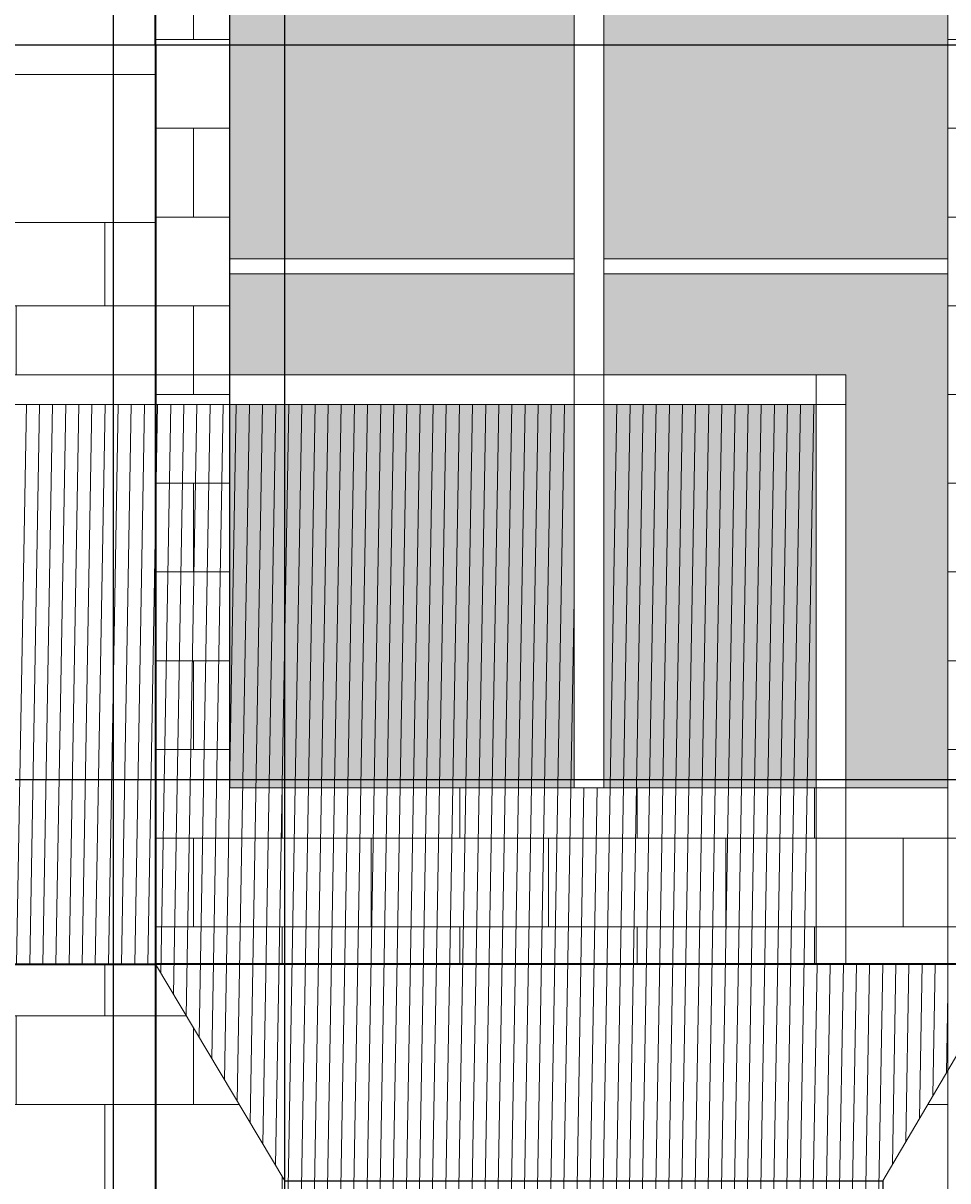
# Model space of a CAD drawing. Units: inches. Extents: x -26 to 776, y -22 to 650.
# Tile 18 of 62: x 222 to 285, y 145 to 223. Entities that reach past the tile are written whole.
import ezdxf

# ---------------------------------------------------------------- set-up
doc = ezdxf.new("R2010")
doc.units = ezdxf.units.IN
doc.header["$MEASUREMENT"] = 0
for name, color, linetype, lineweight in [('A-ANNO-DIMS', 2, 'Continuous', 18), ('A-DETL-PATT', 8, 'Continuous', 13), ('A-DOOR', 3, 'Continuous', 25), ('A-GLAZ', 4, 'Continuous', 18), ('A-GLAZ-PATT', 9, 'Continuous', 13), ('A-WALL', 7, 'Continuous', 35), ('A-WALL-PATT', 8, 'Continuous', 13), ('A-WALL-TRIM', 7, 'Continuous', 18)]:
    doc.layers.add(name, color=color, linetype=linetype, lineweight=lineweight)
doc.styles.get("Standard").update_dxf_attribs({"font": 'arial.ttf'})
doc.dimstyles.get("Standard").update_dxf_attribs({"dimtxt": 0.5625, "dimasz": 0.18, "dimexe": 0.18, "dimexo": 0.0625, "dimgap": 0.09, "dimtad": 0, "dimtih": 1, "dimtoh": 1, "dimdec": 4, "dimzin": 0, "dimdsep": 46, "dimlunit": 4, "dimtxsty": 'Standard', "dimcen": 0.09, "dimadec": 0, "dimazin": 0, "dimtfac": 1, "dimtdec": 4, "dimtofl": 0, "dimtmove": 0, "dimatfit": 3, "dimfxl": 1, "dimtolj": 1, "dimtzin": 0, "dimarcsym": 0})

# ---------------------------------------------------------------- blocks, each defined once
blk = doc.blocks.new('WIN-ELEV-2X4-HEAD')
for p, q in [((23.276, 0), (23.276, 123)), ((25.276, 0), (25.276, 123)), ((0, 35.757), (23.276, 35.757)), ((25.276, 35.757), (48.553, 35.757)), ((0, 34.757), (23.276, 34.757)), ((25.276, 34.757), (48.553, 34.757))]:
    blk.add_line(p, q)
blk.add_lwpolyline([(48.553, 0), (0, 0), (0, 123), (48.553, 123)], close=True)
blk = doc.blocks.new('*D26')
at = {"layer": 'A-ANNO-DIMS', "color": 0, "lineweight": -2, "transparency": 16777216}
for p, q in [((91.707, 171.973), (775.335, 171.973)), ((775.155, 171.793), (775.155, 166.105)), ((775.155, 159.662), (775.155, 165.351)), ((82.196, 159.482), (775.335, 159.482))]:
    blk.add_line(p, q, dxfattribs=at)
at = {"layer": 'A-ANNO-DIMS', "color": 0, "transparency": 16777216}
for points in [[(775.125, 171.793), (775.185, 171.793), (775.155, 171.973)], [(775.125, 159.662), (775.185, 159.662), (775.155, 159.482)]]:
    blk.add_solid(points, dxfattribs=at)
at = {"layer": 'Defpoints', "color": 0, "transparency": 16777216}
for p in [(91.645, 171.973), (775.155, 171.973), (82.134, 159.482)]:
    blk.add_point(p, dxfattribs=at)
at = {"layer": 'A-ANNO-DIMS', "color": 0, "transparency": 16777216, "insert": (775.155, 165.728), "char_height": 0.5625, "attachment_point": 5}
blk.add_mtext('\\A1;12.49', dxfattribs=at)
blk = doc.blocks.new('*D34')
at = {"layer": 'A-ANNO-DIMS', "color": 0, "lineweight": -2, "transparency": 16777216}
for p, q in [((228.573, 528.296), (228.573, -21.315)), ((357.303, 528.361), (357.303, -21.315)), ((228.753, -21.135), (291.707, -21.135)), ((357.123, -21.135), (294.17, -21.135))]:
    blk.add_line(p, q, dxfattribs=at)
at = {"layer": 'A-ANNO-DIMS', "color": 0, "transparency": 16777216}
for points in [[(228.753, -21.105), (228.753, -21.165), (228.573, -21.135)], [(357.123, -21.105), (357.123, -21.165), (357.303, -21.135)]]:
    blk.add_solid(points, dxfattribs=at)
at = {"layer": 'Defpoints', "color": 0, "transparency": 16777216}
for p in [(357.303, 528.423), (228.573, 528.358), (357.303, -21.135)]:
    blk.add_point(p, dxfattribs=at)
at = {"layer": 'A-ANNO-DIMS', "color": 0, "transparency": 16777216, "insert": (292.938, -21.135), "char_height": 0.5625, "attachment_point": 5}
blk.add_mtext('\\A1;128.73', dxfattribs=at)
blk = doc.blocks.new('*D37')
at = {"layer": 'A-ANNO-DIMS', "color": 0, "lineweight": -2, "transparency": 16777216}
for p, q in [((231.362, 159.482), (-25.478, 159.482)), ((-25.298, 159.302), (-25.298, 87.855)), ((-25.298, 15.662), (-25.298, 87.11)), ((217.89, 15.482), (-25.478, 15.482))]:
    blk.add_line(p, q, dxfattribs=at)
at = {"layer": 'A-ANNO-DIMS', "color": 0, "transparency": 16777216}
for points in [[(-25.328, 159.302), (-25.268, 159.302), (-25.298, 159.482)], [(-25.328, 15.662), (-25.268, 15.662), (-25.298, 15.482)]]:
    blk.add_solid(points, dxfattribs=at)
at = {"layer": 'Defpoints', "color": 0, "transparency": 16777216}
for p in [(-25.298, 159.482), (231.425, 159.482), (217.953, 15.482)]:
    blk.add_point(p, dxfattribs=at)
at = {"layer": 'A-ANNO-DIMS', "color": 0, "transparency": 16777216, "insert": (-25.298, 87.482), "char_height": 0.5625, "attachment_point": 5}
blk.add_mtext('\\A1;144', dxfattribs=at)
blk = doc.blocks.new('*D41')
at = {"layer": 'A-ANNO-DIMS', "color": 0, "lineweight": -2, "transparency": 16777216}
for p, q in [((11.17, 221.641), (775.335, 221.641)), ((775.155, 221.461), (775.155, 190.939)), ((775.155, 159.662), (775.155, 190.185)), ((11.17, 159.482), (775.335, 159.482))]:
    blk.add_line(p, q, dxfattribs=at)
at = {"layer": 'A-ANNO-DIMS', "color": 0, "transparency": 16777216}
for points in [[(775.125, 221.461), (775.185, 221.461), (775.155, 221.641)], [(775.125, 159.662), (775.185, 159.662), (775.155, 159.482)]]:
    blk.add_solid(points, dxfattribs=at)
at = {"layer": 'Defpoints', "color": 0, "transparency": 16777216}
for p in [(11.107, 221.641), (775.155, 221.641), (11.107, 159.482)]:
    blk.add_point(p, dxfattribs=at)
at = {"layer": 'A-ANNO-DIMS', "color": 0, "transparency": 16777216, "insert": (775.155, 190.562), "char_height": 0.5625, "attachment_point": 5}
blk.add_mtext('\\A1;62.16', dxfattribs=at)
blk = doc.blocks.new('*D43')
at = {"layer": 'A-ANNO-DIMS', "color": 0, "lineweight": -2, "transparency": 16777216}
for p, q in [((231.425, 159.545), (231.425, 649.856)), ((236.465, 171.48), (236.465, 649.856)), ((231.605, 649.676), (233.125, 649.676)), ((236.285, 649.676), (234.764, 649.676))]:
    blk.add_line(p, q, dxfattribs=at)
at = {"layer": 'A-ANNO-DIMS', "color": 0, "transparency": 16777216}
for points in [[(231.605, 649.706), (231.605, 649.646), (231.425, 649.676)], [(236.285, 649.706), (236.285, 649.646), (236.465, 649.676)]]:
    blk.add_solid(points, dxfattribs=at)
at = {"layer": 'Defpoints', "color": 0, "transparency": 16777216}
for p in [(236.465, 649.676), (236.465, 171.417), (231.425, 159.482)]:
    blk.add_point(p, dxfattribs=at)
at = {"layer": 'A-ANNO-DIMS', "color": 0, "transparency": 16777216, "insert": (233.945, 649.676), "char_height": 0.5625, "attachment_point": 5}
blk.add_mtext('\\A1;5.04', dxfattribs=at)
blk = doc.blocks.new('*D44')
at = {"layer": 'A-ANNO-DIMS', "color": 0, "lineweight": -2, "transparency": 16777216}
for p, q in [((231.425, 15.545), (231.425, 649.856)), ((240.165, 26.486), (240.165, 649.856)), ((231.605, 649.676), (234.975, 649.676)), ((239.985, 649.676), (236.615, 649.676))]:
    blk.add_line(p, q, dxfattribs=at)
at = {"layer": 'A-ANNO-DIMS', "color": 0, "transparency": 16777216}
for points in [[(231.605, 649.706), (231.605, 649.646), (231.425, 649.676)], [(239.985, 649.706), (239.985, 649.646), (240.165, 649.676)]]:
    blk.add_solid(points, dxfattribs=at)
at = {"layer": 'Defpoints', "color": 0, "transparency": 16777216}
for p in [(240.165, 649.676), (240.165, 26.424), (231.425, 15.482)]:
    blk.add_point(p, dxfattribs=at)
at = {"layer": 'A-ANNO-DIMS', "color": 0, "transparency": 16777216, "insert": (235.795, 649.676), "char_height": 0.5625, "attachment_point": 5}
blk.add_mtext('\\A1;8.74', dxfattribs=at)

msp = doc.modelspace()

# ---------------------------------------------------------------- hatches: boundary and pattern name
at = {"layer": 'A-DETL-PATT'}
h = msp.add_hatch(dxfattribs=at)
h.set_pattern_fill('ANSI31', color=256, scale=7.1, angle=44)
h.paths.add_polyline_path([(231.4249, 197.3298), (216.1056, 197.3298), (216.1056, 159.4824), (231.4249, 159.4824)])
h.paths.add_polyline_path([(236.4647, 197.3298), (231.4249, 197.3298), (231.4249, 159.4824), (276.1134, 159.4824), (276.1134, 171.4173), (236.4647, 171.4173)])
h.paths.add_polyline_path([(259.7413, 197.3298), (236.4647, 197.3298), (236.4647, 171.4173), (259.7413, 171.4173)], flags=17)
h.paths.add_polyline_path([(276.1134, 197.3298), (261.7413, 197.3298), (261.7413, 171.4173), (276.1134, 171.4173)], flags=17)
h.paths.add_polyline_path([(217.9529, 147.0781), (22.8891, 147.0781), (22.8891, 138.3844), (217.9529, 138.3844)])
h.paths.add_polyline_path([(285.0179, 152.3087), (285.0179, 159.4824), (231.4249, 159.4824), (240.1654, 144.8359), (280.6173, 144.8359)])
h.paths.add_polyline_path([(280.6173, 144.8359), (240.1654, 144.8359), (240.1654, 26.4239), (280.6173, 26.4239)])
h.paths.add_polyline_path([(274.6644, 134.8811), (274.6644, 34.0885), (245.7207, 34.0885), (245.7207, 134.8811)], flags=16)
h.paths.add_polyline_path([(285.0179, 303.3046), (236.4647, 303.3046), (236.4647, 294.4171), (285.0179, 294.4171)])
h.paths.add_polyline_path([(285.0179, 446.0063), (236.4647, 446.0063), (236.4647, 437.1188), (285.0179, 437.1188)])
at = {"layer": 'A-GLAZ-PATT'}
h = msp.add_hatch(dxfattribs=at)
h.set_pattern_fill('GOST_GLASS', color=256, scale=0.75)
h.set_pattern_definition([(45, (0, 0), (6.36396, 0), [3.75, -5.25]), (45, (1.591, 0), (6.36396, 0), [1.5, -7.5]), (45, (0, 1.591), (6.36396, 0), [1.5, -7.5])])
h.paths.add_polyline_path([(115.8402, 198.8773), (93.6448, 198.8773), (93.6448, 173.9734), (115.8402, 173.9734)])
h.paths.add_polyline_path([(144.1571, 198.8773), (115.8402, 198.8773), (115.8402, 173.9734), (144.1571, 173.9734)])
h.paths.add_polyline_path([(115.8402, 224.3396), (93.6448, 224.3396), (93.6448, 198.8773), (115.8402, 198.8773)])
h.paths.add_polyline_path([(144.1571, 248.4417), (115.8402, 248.4417), (115.8402, 224.3396), (144.1571, 224.3396)])
h.paths.add_polyline_path([(144.1571, 224.3396), (115.8402, 224.3396), (115.8402, 198.8773), (144.1571, 198.8773)])
h.paths.add_polyline_path([(170.5449, 224.3396), (144.1571, 224.3396), (144.1571, 198.8773), (170.5449, 198.8773)])
h.paths.add_polyline_path([(170.5449, 198.8773), (144.1571, 198.8773), (144.1571, 173.9734), (170.5449, 173.9734)])
h.paths.add_polyline_path([(194.6694, 198.8773), (170.5449, 198.8773), (170.5449, 173.9734), (194.6694, 173.9734)])
h.paths.add_polyline_path([(194.6694, 224.3396), (170.5449, 224.3396), (170.5449, 198.8773), (194.6694, 198.8773)])
h.paths.add_polyline_path([(194.6694, 248.4417), (170.5449, 248.4417), (170.5449, 224.3396), (194.6694, 224.3396)])
h.paths.add_polyline_path([(170.5449, 248.4417), (144.1571, 248.4417), (144.1571, 224.3396), (170.5449, 224.3396)])
h.paths.add_polyline_path([(144.1571, 269.3091), (115.8402, 269.3091), (115.8402, 248.4417), (144.1571, 248.4417)])
h.paths.add_polyline_path([(115.8402, 269.3091), (93.6448, 269.3091), (93.6448, 248.4417), (115.8402, 248.4417)])
h.paths.add_polyline_path([(115.8402, 248.4417), (93.6448, 248.4417), (93.6448, 224.3396), (115.8402, 224.3396)])
h.paths.add_polyline_path([(170.5449, 269.3091), (144.1571, 269.3091), (144.1571, 248.4417), (170.5449, 248.4417)])
h.paths.add_polyline_path([(194.6694, 269.3091), (170.5449, 269.3091), (170.5449, 248.4417), (194.6694, 248.4417)])
h.paths.add_polyline_path([(259.7413, 294.4171), (236.4647, 294.4171), (236.4647, 266.1888), (259.7413, 266.1888)])
h.paths.add_polyline_path([(285.0179, 294.4171), (261.7413, 294.4171), (261.7413, 266.1888), (285.0179, 266.1888)])
h.paths.add_polyline_path([(285.0179, 265.1888), (261.7413, 265.1888), (261.7413, 233.9172), (285.0179, 233.9172)])
h.paths.add_polyline_path([(259.7413, 265.1888), (236.4647, 265.1888), (236.4647, 233.9172), (259.7413, 233.9172)])
h.paths.add_polyline_path([(259.7413, 232.9172), (236.4647, 232.9172), (236.4647, 207.1741), (259.7413, 207.1741)])
h.paths.add_polyline_path([(285.0179, 232.9172), (261.7413, 232.9172), (261.7413, 207.1741), (285.0179, 207.1741)])
h.paths.add_polyline_path([(285.0179, 206.1741), (261.7413, 206.1741), (261.7413, 199.3298), (278.1134, 199.3298), (278.1134, 171.4173), (285.0179, 171.4173)])
h.paths.add_polyline_path([(259.7413, 206.1741), (236.4647, 206.1741), (236.4647, 199.3298), (259.7413, 199.3298)])
h.paths.add_polyline_path([(259.7413, 197.3298), (236.4647, 197.3298), (236.4647, 171.4173), (259.7413, 171.4173)])
h.paths.add_polyline_path([(276.1134, 197.3298), (261.7413, 197.3298), (261.7413, 171.4173), (276.1134, 171.4173)], flags=17)
h.paths.add_polyline_path([(255.8125, 548.0348), (228.5733, 548.0348), (228.5733, 528.3585), (255.8125, 528.3585)])
h.paths.add_polyline_path([(281.6181, 548.0348), (256.0792, 548.0348), (256.0792, 528.3585), (281.6181, 528.3585)])
h.paths.add_polyline_path([(308.8797, 548.0348), (281.789, 548.0348), (281.789, 528.3585), (308.8797, 528.3585)])
h.paths.add_polyline_path([(357.2724, 548.0995), (309.2457, 548.0348), (309.2457, 528.3585), (357.3034, 528.4233), (357.3034, 538.2614)])
h.paths.add_polyline_path([(259.7413, 437.1188), (236.4647, 437.1188), (236.4647, 408.8905), (259.7413, 408.8905)])
h.paths.add_polyline_path([(285.0179, 437.1188), (261.7413, 437.1188), (261.7413, 408.8905), (285.0179, 408.8905)])
h.paths.add_polyline_path([(259.7413, 407.8905), (236.4647, 407.8905), (236.4647, 376.6189), (259.7413, 376.6189)])
h.paths.add_polyline_path([(285.0179, 407.8905), (261.7413, 407.8905), (261.7413, 376.6189), (285.0179, 376.6189)])
h.paths.add_polyline_path([(285.0179, 375.6189), (261.7413, 375.6189), (261.7413, 349.8758), (285.0179, 349.8758)])
h.paths.add_polyline_path([(285.0179, 348.8758), (261.7413, 348.8758), (261.7413, 314.119), (285.0179, 314.119)])
h.paths.add_polyline_path([(259.7413, 348.8758), (236.4647, 348.8758), (236.4647, 314.119), (259.7413, 314.119)])
h.paths.add_polyline_path([(259.7413, 375.6189), (236.4647, 375.6189), (236.4647, 349.8758), (259.7413, 349.8758)])
h.paths.add_polyline_path([(194.6694, 404.1909), (170.5449, 404.1909), (170.5449, 383.3235), (194.6694, 383.3235)])
h.paths.add_polyline_path([(170.5449, 404.1909), (144.1571, 404.1909), (144.1571, 383.3235), (170.5449, 383.3235)])
h.paths.add_polyline_path([(144.1571, 404.1909), (115.8402, 404.1909), (115.8402, 383.3235), (144.1571, 383.3235)])
h.paths.add_polyline_path([(115.8402, 404.1909), (93.6448, 404.1909), (93.6448, 383.3235), (115.8402, 383.3235)])
h.paths.add_polyline_path([(115.8402, 383.3235), (93.6448, 383.3235), (93.6448, 359.2214), (115.8402, 359.2214)])
h.paths.add_polyline_path([(144.1571, 383.3235), (115.8402, 383.3235), (115.8402, 359.2214), (144.1571, 359.2214)])
h.paths.add_polyline_path([(115.8402, 359.2214), (93.6448, 359.2214), (93.6448, 333.7591), (115.8402, 333.7591)])
h.paths.add_polyline_path([(144.1571, 359.2214), (115.8402, 359.2214), (115.8402, 333.7591), (144.1571, 333.7591)])
h.paths.add_polyline_path([(115.8402, 333.7591), (93.6448, 333.7591), (93.6448, 308.8552), (115.8402, 308.8552)])
h.paths.add_polyline_path([(144.1571, 333.7591), (115.8402, 333.7591), (115.8402, 308.8552), (144.1571, 308.8552)])
h.paths.add_polyline_path([(170.5449, 333.7591), (144.1571, 333.7591), (144.1571, 308.8552), (170.5449, 308.8552)])
h.paths.add_polyline_path([(170.5449, 359.2214), (144.1571, 359.2214), (144.1571, 333.7591), (170.5449, 333.7591)])
h.paths.add_polyline_path([(170.5449, 383.3235), (144.1571, 383.3235), (144.1571, 359.2214), (170.5449, 359.2214)])
h.paths.add_polyline_path([(194.6694, 383.3235), (170.5449, 383.3235), (170.5449, 359.2214), (194.6694, 359.2214)])
h.paths.add_polyline_path([(194.6694, 359.2214), (170.5449, 359.2214), (170.5449, 333.7591), (194.6694, 333.7591)])
h.paths.add_polyline_path([(194.6694, 333.7591), (170.5449, 333.7591), (170.5449, 308.8552), (194.6694, 308.8552)])
at = {"layer": 'A-WALL-PATT'}
h = msp.add_hatch(dxfattribs=at)
h.set_pattern_fill('AR-B816', color=256, scale=0.75)
h.paths.add_polyline_path([(289.2424, 504.4205), (231.4249, 504.4205), (231.4249, 458.1203), (231.4249, 221.6413), (231.4249, 209.6413), (231.4249, 159.4824), (285.0179, 159.4824), (285.0179, 171.4173), (236.4647, 171.4173), (236.4647, 294.4171), (236.4647, 303.3046), (285.0179, 303.3046), (285.0179, 294.4171), (285.0179, 171.4173), (285.0179, 159.4824), (289.2424, 159.4824), (289.2424, 291.1798), (289.2424, 458.1203)])
h.paths.add_polyline_path([(285.0179, 446.0063), (285.0179, 437.1188), (285.0179, 314.119), (236.4647, 314.119), (236.4647, 437.1188), (236.4647, 446.0063)], flags=16)
h = msp.add_hatch(dxfattribs=at)
h.set_pattern_fill('AR-B816', color=256, scale=0.75)
h.paths.add_polyline_path([(82.134, 209.6413), (11.1074, 209.6413), (11.1074, 159.4824), (82.134, 159.4824)])
h.paths.add_polyline_path([(231.4249, 209.6413), (209.091, 209.6413), (209.091, 159.4824), (214.1056, 159.4824), (214.1056, 199.3298), (231.4249, 199.3298)])
h.paths.add_polyline_path([(231.4249, 159.4824), (11.1074, 159.4824), (11.1074, 22.5014), (22.8891, 22.5014), (22.8891, 147.0781), (217.9529, 147.0781), (217.9529, 20.7937), (231.4249, 20.7937)])
h.paths.add_polyline_path([(285.0179, 152.3087), (280.6173, 144.8359), (280.6173, 26.4239), (240.1654, 26.4239), (240.1654, 144.8359), (231.4249, 159.4824), (231.4249, 20.7937), (285.0179, 20.7937)])

# ---------------------------------------------------------------- linework, layer by layer
at = {"layer": 'A-DOOR'}
msp.add_lwpolyline([(240.1654, 144.8359), (280.6173, 144.8359), (280.6173, 26.4239), (240.1654, 26.4239)], close=True, dxfattribs=at)
at = {"layer": 'A-WALL'}
for p, q in [((231.4249, 221.6413), (231.4249, 458.1203)), ((231.4249, 221.6413), (231.4249, 209.6413)), ((231.4249, 209.6413), (231.4249, 159.4824)), ((11.1074, 159.4824), (231.4249, 159.4824)), ((231.4249, 159.4824), (231.4249, 15.4824)), ((289.2424, 159.4824), (231.4249, 159.4824))]:
    msp.add_line(p, q, dxfattribs=at)
at = {"layer": 'A-WALL-TRIM'}
for p, q in [((285.0179, 15.4824), (285.0179, 249.6598)), ((209.091, 221.6413), (231.4249, 221.6413)), ((209.091, 219.6413), (231.4249, 219.6413)), ((209.091, 209.6413), (231.4249, 209.6413)), ((214.1056, 199.3298), (278.1134, 199.3298)), ((276.1134, 199.3298), (276.1134, 159.4824)), ((278.1134, 199.3298), (278.1134, 159.4824)), ((214.1056, 197.3298), (278.1134, 197.3298)), ((240.1654, 144.8359), (231.4249, 159.4824)), ((280.6173, 144.8359), (289.2424, 159.4824))]:
    msp.add_line(p, q, dxfattribs=at)

# ---------------------------------------------------------------- block references
at = {"layer": 'A-GLAZ'}
msp.add_blockref('WIN-ELEV-2X4-HEAD', (236.465, 171.417), dxfattribs=at)

# ---------------------------------------------------------------- dimensions: what is measured, and where the dimension line sits
at = {"layer": 'A-ANNO-DIMS'}
for base, p1, p2, picture, middle in [((236.4647, 649.6763), (231.4249, 159.4824), (236.4647, 171.4173), '*D43', (233.9448, 649.6763)), ((240.1654, 649.6763), (231.4249, 15.4824), (240.1654, 26.4239), '*D44', (235.7952, 649.6763)), ((357.3034, -21.1349), (228.5733, 528.3585), (357.3034, 528.4233), '*D34', (292.9384, -21.1349))]:
    dim = msp.add_linear_dim(base=base, p1=p1, p2=p2, dimstyle='Standard', override={"dimdec": 2, "dimlfac": 1, "dimrnd": 0, "dimzin": 0, "dimdsep": 46, "dimlunit": 2}, dxfattribs=at)
    dim.commit()
    dim.dimension.update_dxf_attribs({"geometry": picture, "text_midpoint": middle})
for base, p1, p2, override, picture, middle in [((775.1553, 221.6413), (11.1074, 159.4824), (11.1074, 221.6413), {"dimdec": 2, "dimlfac": 1, "dimrnd": 0, "dimzin": 0, "dimdsep": 46, "dimlunit": 2}, '*D41', (775.1553, 190.5618)), ((775.1553, 171.9734), (82.134, 159.4824), (91.6448, 171.9734), {"dimdec": 2, "dimlfac": 1, "dimrnd": 0, "dimzin": 0, "dimdsep": 46, "dimlunit": 2}, '*D26', (775.1553, 165.7279)), ((-25.2976, 159.4824), (217.9529, 15.4824), (231.4249, 159.4824), {"dimdec": 0, "dimlfac": 1, "dimrnd": 0, "dimzin": 0, "dimdsep": 46, "dimlunit": 2}, '*D37', (-25.2976, 87.4824))]:
    dim = msp.add_linear_dim(base=base, p1=p1, p2=p2, angle=90, dimstyle='Standard', override=override, dxfattribs=at)
    dim.commit()
    dim.dimension.update_dxf_attribs({"geometry": picture, "text_midpoint": middle})

doc.saveas('drawing.dxf')
